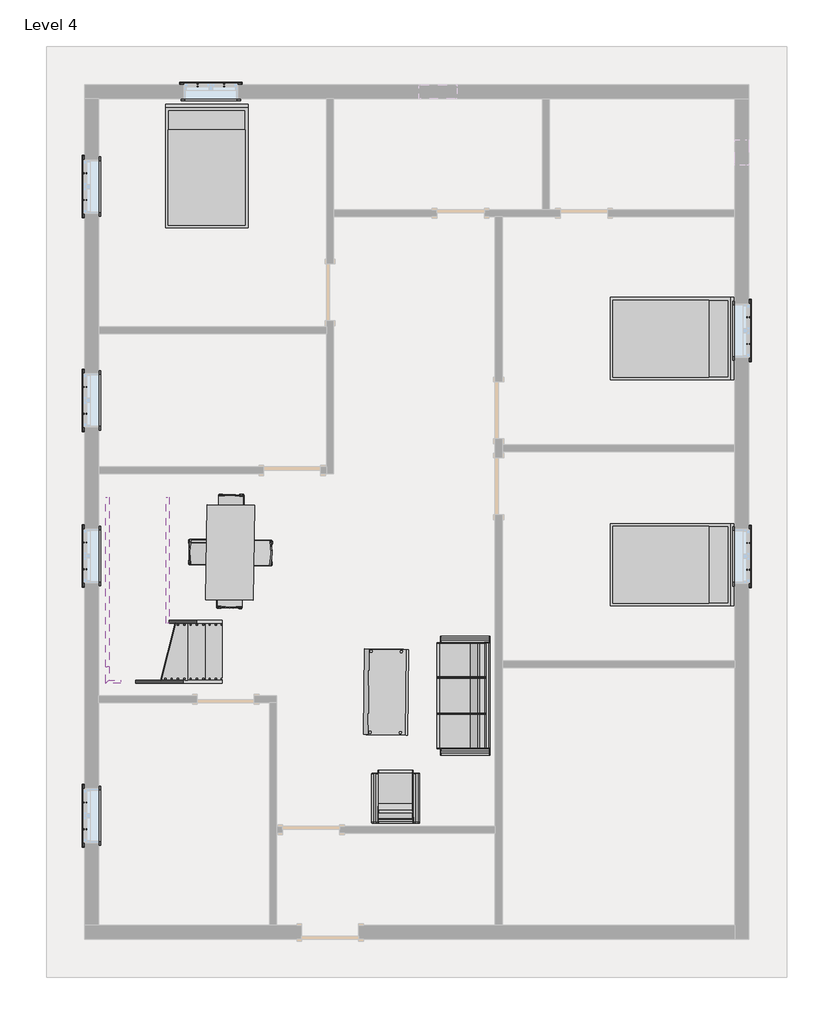
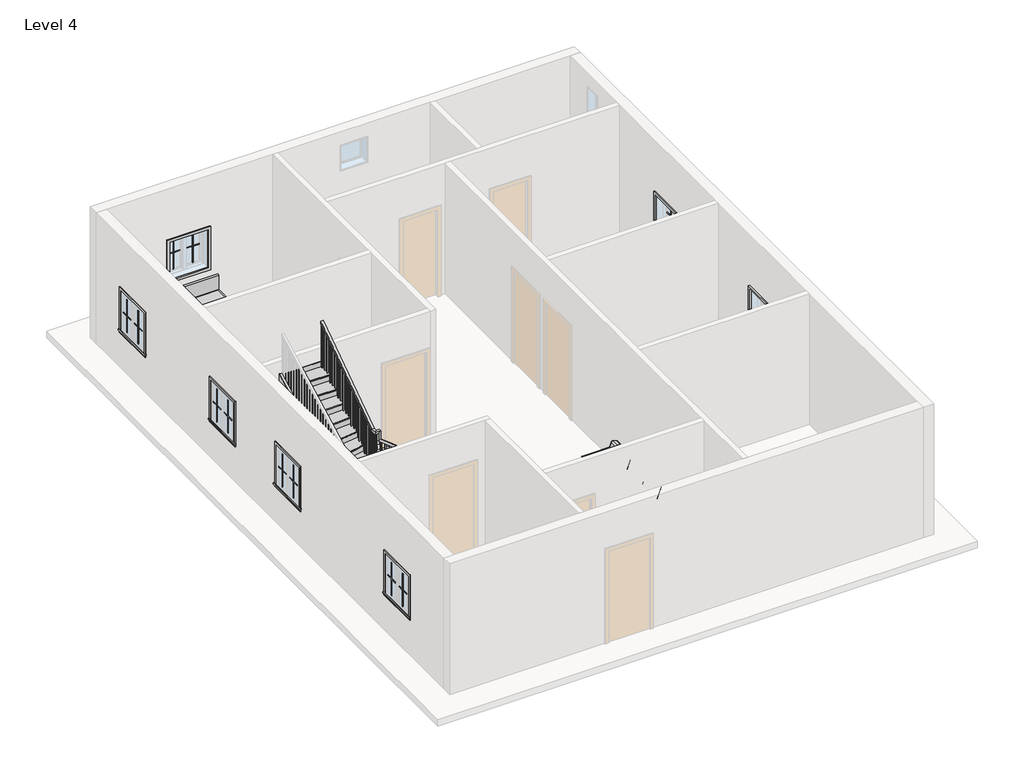
# One storey, part 2 of 2: 29 proxies, 6 furniture elements, 6 members, 1 railing, 1 stair flight.
"""IFC4 building model written with IfcOpenShell, lengths in millimetres."""

from ifc_helpers import new_model, si_unit, frame, origin, place, context, project, spatial, polyline, outline, extrude, faceted_brep, transform, mapped, element, save
from components import modern_coffee_table_17989_modern_coffee_table_17989_d3a860c8, muntin_pattern_2x2_muntin_pattern_2x2_b3fe6957, muntin_pattern_2x2_muntin_pattern_2x2_3e0ecaf2, trim_window_exterior_flat_with_sill_41619996, trim_window_interior_flat_picture_frame_51c85655, furniture_2fc85b74, furniture_29a9adb8, furniture_57072a26, furniture_f28dd14e, furniture_402a1f5e, bed_17739_bed_17739_15c61121, dining_table_w_chairs_11374_0cdfc61b, stair_flight_62476df0

model = new_model("IFC4")

# Units and contexts
model_context = context("Model", 3, world=origin())
ifc_project = project(units=[si_unit("LENGTHUNIT", "METRE", prefix="MILLI")], contexts=[model_context])

# Site, building, storey
site = spatial("IfcSite", under=ifc_project)
building = spatial("IfcBuilding", under=site)
storey = spatial("IfcBuildingStorey", under=building, Name="Level 4", Elevation=6400.8)

# Proxies
placement = place(None, origin())
modern_coffee_table_17989_modern_coffee_table_17989_shape = modern_coffee_table_17989_modern_coffee_table_17989_d3a860c8(model_context)
element("IfcBuildingElementProxy", 1, Name="Modern_Coffee_Table_17989 : Modern_Coffee_Table_17989", ObjectType="Modern_Coffee_Table_17989 : Modern_Coffee_Table_17989", at=placement, inside=storey, context=model_context, shape_type="MappedRepresentation", body=[
    mapped(modern_coffee_table_17989_modern_coffee_table_17989_shape, transform((-2106.8718825, -2116.758017, 6400.8), x_axis=(0.012591066442684793, 0.9999207293810025, 0.0), y_axis=(-0.9999207293810025, 0.012591066442684793, 0.0), z_axis=(0.0, 0.0, 1.0))),
])
muntin_pattern_2x2_muntin_pattern_2x2_shape = muntin_pattern_2x2_muntin_pattern_2x2_b3fe6957(model_context)
element("IfcBuildingElementProxy", 2, Name="Muntin Pattern_2x2 : Muntin Pattern_2x2", ObjectType="Muntin Pattern_2x2 : Muntin Pattern_2x2", at=placement, inside=storey, context=model_context, shape_type="MappedRepresentation", body=[
    mapped(muntin_pattern_2x2_muntin_pattern_2x2_shape, transform((-4775.9474931, 7386.6685985, 7385.05), x_axis=(1.0, 0.0, 0.0), y_axis=(0.0, 1.0, 0.0), z_axis=(0.0, 0.0, 1.0))),
])
element("IfcBuildingElementProxy", 3, Name="Muntin Pattern_2x2 : Muntin Pattern_2x2", ObjectType="Muntin Pattern_2x2 : Muntin Pattern_2x2", at=placement, inside=storey, context=model_context, shape_type="MappedRepresentation", body=[
    mapped(muntin_pattern_2x2_muntin_pattern_2x2_shape, transform((4068.0150069, 3660.8060985, 7385.05), x_axis=(0.0, -1.0, 0.0), y_axis=(1.0, 0.0, 0.0), z_axis=(0.0, 0.0, 1.0))),
])
element("IfcBuildingElementProxy", 4, Name="Muntin Pattern_2x2 : Muntin Pattern_2x2", ObjectType="Muntin Pattern_2x2 : Muntin Pattern_2x2", at=placement, inside=storey, context=model_context, shape_type="MappedRepresentation", body=[
    mapped(muntin_pattern_2x2_muntin_pattern_2x2_shape, transform((4068.0150069, 40.9802908, 7385.05), x_axis=(0.0, -1.0, 0.0), y_axis=(1.0, 0.0, 0.0), z_axis=(0.0, 0.0, 1.0))),
])
element("IfcBuildingElementProxy", 5, Name="Muntin Pattern_2x2 : Muntin Pattern_2x2", ObjectType="Muntin Pattern_2x2 : Muntin Pattern_2x2", at=placement, inside=storey, context=model_context, shape_type="MappedRepresentation", body=[
    mapped(muntin_pattern_2x2_muntin_pattern_2x2_shape, transform((-6580.9349931, 2114.5810985, 7385.05), x_axis=(0.0, 1.0, 0.0), y_axis=(-1.0, 0.0, 0.0), z_axis=(0.0, 0.0, 1.0))),
])
element("IfcBuildingElementProxy", 6, Name="Muntin Pattern_2x2 : Muntin Pattern_2x2", ObjectType="Muntin Pattern_2x2 : Muntin Pattern_2x2", at=placement, inside=storey, context=model_context, shape_type="MappedRepresentation", body=[
    mapped(muntin_pattern_2x2_muntin_pattern_2x2_shape, transform((-6580.9349931, 5543.5810985, 7385.05), x_axis=(0.0, 1.0, 0.0), y_axis=(-1.0, 0.0, 0.0), z_axis=(0.0, 0.0, 1.0))),
])
element("IfcBuildingElementProxy", 7, Name="Muntin Pattern_2x2 : Muntin Pattern_2x2", ObjectType="Muntin Pattern_2x2 : Muntin Pattern_2x2", at=placement, inside=storey, context=model_context, shape_type="MappedRepresentation", body=[
    mapped(muntin_pattern_2x2_muntin_pattern_2x2_shape, transform((-6580.9349931, -4549.7439015, 7385.05), x_axis=(0.0, 1.0, 0.0), y_axis=(-1.0, 0.0, 0.0), z_axis=(0.0, 0.0, 1.0))),
])
element("IfcBuildingElementProxy", 8, Name="Muntin Pattern_2x2 : Muntin Pattern_2x2", ObjectType="Muntin Pattern_2x2 : Muntin Pattern_2x2", at=placement, inside=storey, context=model_context, shape_type="MappedRepresentation", body=[
    mapped(muntin_pattern_2x2_muntin_pattern_2x2_shape, transform((-6580.9349931, -380.9689015, 7385.05), x_axis=(0.0, 1.0, 0.0), y_axis=(-1.0, 0.0, 0.0), z_axis=(0.0, 0.0, 1.0))),
])
muntin_pattern_2x2_muntin_pattern_2x2_2_shape = muntin_pattern_2x2_muntin_pattern_2x2_3e0ecaf2(model_context)
element("IfcBuildingElementProxy", 9, Name="Muntin Pattern_2x2 : Muntin Pattern_2x2", ObjectType="Muntin Pattern_2x2 : Muntin Pattern_2x2", at=placement, inside=storey, context=model_context, shape_type="MappedRepresentation", body=[
    mapped(muntin_pattern_2x2_muntin_pattern_2x2_2_shape, transform((-4347.3224931, 7386.6685985, 7385.05), x_axis=(-1.0, 0.0, 0.0), y_axis=(0.0, -1.0, 0.0), z_axis=(0.0, 0.0, 1.0))),
])
element("IfcBuildingElementProxy", 10, Name="Muntin Pattern_2x2 : Muntin Pattern_2x2", ObjectType="Muntin Pattern_2x2 : Muntin Pattern_2x2", at=placement, inside=storey, context=model_context, shape_type="MappedRepresentation", body=[
    mapped(muntin_pattern_2x2_muntin_pattern_2x2_2_shape, transform((4068.0150069, 3232.1810985, 7385.05), x_axis=(0.0, 1.0, 0.0), y_axis=(-1.0, 0.0, 0.0), z_axis=(0.0, 0.0, 1.0))),
])
element("IfcBuildingElementProxy", 11, Name="Muntin Pattern_2x2 : Muntin Pattern_2x2", ObjectType="Muntin Pattern_2x2 : Muntin Pattern_2x2", at=placement, inside=storey, context=model_context, shape_type="MappedRepresentation", body=[
    mapped(muntin_pattern_2x2_muntin_pattern_2x2_2_shape, transform((4068.0150069, -387.6447092, 7385.05), x_axis=(0.0, 1.0, 0.0), y_axis=(-1.0, 0.0, 0.0), z_axis=(0.0, 0.0, 1.0))),
])
element("IfcBuildingElementProxy", 12, Name="Muntin Pattern_2x2 : Muntin Pattern_2x2", ObjectType="Muntin Pattern_2x2 : Muntin Pattern_2x2", at=placement, inside=storey, context=model_context, shape_type="MappedRepresentation", body=[
    mapped(muntin_pattern_2x2_muntin_pattern_2x2_2_shape, transform((-6580.9349931, 2543.2060985, 7385.05), x_axis=(0.0, -1.0, 0.0), y_axis=(1.0, 0.0, 0.0), z_axis=(0.0, 0.0, 1.0))),
])
element("IfcBuildingElementProxy", 13, Name="Muntin Pattern_2x2 : Muntin Pattern_2x2", ObjectType="Muntin Pattern_2x2 : Muntin Pattern_2x2", at=placement, inside=storey, context=model_context, shape_type="MappedRepresentation", body=[
    mapped(muntin_pattern_2x2_muntin_pattern_2x2_2_shape, transform((-6580.9349931, 5972.2060985, 7385.05), x_axis=(0.0, -1.0, 0.0), y_axis=(1.0, 0.0, 0.0), z_axis=(0.0, 0.0, 1.0))),
])
element("IfcBuildingElementProxy", 14, Name="Muntin Pattern_2x2 : Muntin Pattern_2x2", ObjectType="Muntin Pattern_2x2 : Muntin Pattern_2x2", at=placement, inside=storey, context=model_context, shape_type="MappedRepresentation", body=[
    mapped(muntin_pattern_2x2_muntin_pattern_2x2_2_shape, transform((-6580.9349931, -4121.1189015, 7385.05), x_axis=(0.0, -1.0, 0.0), y_axis=(1.0, 0.0, 0.0), z_axis=(0.0, 0.0, 1.0))),
])
element("IfcBuildingElementProxy", 15, Name="Muntin Pattern_2x2 : Muntin Pattern_2x2", ObjectType="Muntin Pattern_2x2 : Muntin Pattern_2x2", at=placement, inside=storey, context=model_context, shape_type="MappedRepresentation", body=[
    mapped(muntin_pattern_2x2_muntin_pattern_2x2_2_shape, transform((-6580.9349931, 47.6560985, 7385.05), x_axis=(0.0, -1.0, 0.0), y_axis=(1.0, 0.0, 0.0), z_axis=(0.0, 0.0, 1.0))),
])
trim_window_exterior_flat_with_sill_shape = trim_window_exterior_flat_with_sill_41619996(model_context)
element("IfcBuildingElementProxy", 16, Name="Trim-Window-Exterior-Flat : with Sill", ObjectType="Trim-Window-Exterior-Flat : with Sill", at=placement, inside=storey, context=model_context, shape_type="MappedRepresentation", body=[
    mapped(trim_window_exterior_flat_with_sill_shape, transform((-4561.6349931, 7396.1935985, 8229.6), x_axis=(-1.0, 0.0, 0.0), y_axis=(0.0, 0.0, 1.0), z_axis=(0.0, 1.0, 0.0))),
])
element("IfcBuildingElementProxy", 17, Name="Trim-Window-Exterior-Flat : with Sill", ObjectType="Trim-Window-Exterior-Flat : with Sill", at=placement, inside=storey, context=model_context, shape_type="MappedRepresentation", body=[
    mapped(trim_window_exterior_flat_with_sill_shape, transform((4077.5400069, 3446.4935985, 8229.6), x_axis=(0.0, 1.0, 0.0), y_axis=(0.0, 0.0, 1.0), z_axis=(1.0, 0.0, 0.0))),
])
element("IfcBuildingElementProxy", 18, Name="Trim-Window-Exterior-Flat : with Sill", ObjectType="Trim-Window-Exterior-Flat : with Sill", at=placement, inside=storey, context=model_context, shape_type="MappedRepresentation", body=[
    mapped(trim_window_exterior_flat_with_sill_shape, transform((4077.5400069, -173.3322092, 8229.6), x_axis=(0.0, 1.0, 0.0), y_axis=(0.0, 0.0, 1.0), z_axis=(1.0, 0.0, 0.0))),
])
element("IfcBuildingElementProxy", 19, Name="Trim-Window-Exterior-Flat : with Sill", ObjectType="Trim-Window-Exterior-Flat : with Sill", at=placement, inside=storey, context=model_context, shape_type="MappedRepresentation", body=[
    mapped(trim_window_exterior_flat_with_sill_shape, transform((-6590.4599931, 2328.8935985, 8229.6), x_axis=(0.0, -1.0, 0.0), y_axis=(0.0, 0.0, 1.0), z_axis=(-1.0, 0.0, 0.0))),
])
element("IfcBuildingElementProxy", 20, Name="Trim-Window-Exterior-Flat : with Sill", ObjectType="Trim-Window-Exterior-Flat : with Sill", at=placement, inside=storey, context=model_context, shape_type="MappedRepresentation", body=[
    mapped(trim_window_exterior_flat_with_sill_shape, transform((-6590.4599931, 5757.8935985, 8229.6), x_axis=(0.0, -1.0, 0.0), y_axis=(0.0, 0.0, 1.0), z_axis=(-1.0, 0.0, 0.0))),
])
element("IfcBuildingElementProxy", 21, Name="Trim-Window-Exterior-Flat : with Sill", ObjectType="Trim-Window-Exterior-Flat : with Sill", at=placement, inside=storey, context=model_context, shape_type="MappedRepresentation", body=[
    mapped(trim_window_exterior_flat_with_sill_shape, transform((-6590.4599931, -4335.4314015, 8229.6), x_axis=(0.0, -1.0, 0.0), y_axis=(0.0, 0.0, 1.0), z_axis=(-1.0, 0.0, 0.0))),
])
element("IfcBuildingElementProxy", 22, Name="Trim-Window-Exterior-Flat : with Sill", ObjectType="Trim-Window-Exterior-Flat : with Sill", at=placement, inside=storey, context=model_context, shape_type="MappedRepresentation", body=[
    mapped(trim_window_exterior_flat_with_sill_shape, transform((-6590.4599931, -166.6564015, 8229.6), x_axis=(0.0, -1.0, 0.0), y_axis=(0.0, 0.0, 1.0), z_axis=(-1.0, 0.0, 0.0))),
])
trim_window_interior_flat_picture_frame_shape = trim_window_interior_flat_picture_frame_51c85655(model_context)
element("IfcBuildingElementProxy", 23, Name="Trim-Window-Interior-Flat : Picture Frame", ObjectType="Trim-Window-Interior-Flat : Picture Frame", at=placement, inside=storey, context=model_context, shape_type="MappedRepresentation", body=[
    mapped(trim_window_interior_flat_picture_frame_shape, transform((-4561.6349931, 7167.5935985, 8229.6), x_axis=(1.0, 0.0, 0.0), y_axis=(0.0, 0.0, 1.0), z_axis=(0.0, -1.0, 0.0))),
])
element("IfcBuildingElementProxy", 24, Name="Trim-Window-Interior-Flat : Picture Frame", ObjectType="Trim-Window-Interior-Flat : Picture Frame", at=placement, inside=storey, context=model_context, shape_type="MappedRepresentation", body=[
    mapped(trim_window_interior_flat_picture_frame_shape, transform((3848.9400069, 3446.4935985, 8229.6), x_axis=(0.0, -1.0, 0.0), y_axis=(0.0, 0.0, 1.0), z_axis=(-1.0, 0.0, 0.0))),
])
element("IfcBuildingElementProxy", 25, Name="Trim-Window-Interior-Flat : Picture Frame", ObjectType="Trim-Window-Interior-Flat : Picture Frame", at=placement, inside=storey, context=model_context, shape_type="MappedRepresentation", body=[
    mapped(trim_window_interior_flat_picture_frame_shape, transform((3848.9400069, -173.3322092, 8229.6), x_axis=(0.0, -1.0, 0.0), y_axis=(0.0, 0.0, 1.0), z_axis=(-1.0, 0.0, 0.0))),
])
element("IfcBuildingElementProxy", 26, Name="Trim-Window-Interior-Flat : Picture Frame", ObjectType="Trim-Window-Interior-Flat : Picture Frame", at=placement, inside=storey, context=model_context, shape_type="MappedRepresentation", body=[
    mapped(trim_window_interior_flat_picture_frame_shape, transform((-6361.8599931, 2328.8935985, 8229.6), x_axis=(0.0, 1.0, 0.0), y_axis=(0.0, 0.0, 1.0), z_axis=(1.0, 0.0, 0.0))),
])
element("IfcBuildingElementProxy", 27, Name="Trim-Window-Interior-Flat : Picture Frame", ObjectType="Trim-Window-Interior-Flat : Picture Frame", at=placement, inside=storey, context=model_context, shape_type="MappedRepresentation", body=[
    mapped(trim_window_interior_flat_picture_frame_shape, transform((-6361.8599931, 5757.8935985, 8229.6), x_axis=(0.0, 1.0, 0.0), y_axis=(0.0, 0.0, 1.0), z_axis=(1.0, 0.0, 0.0))),
])
element("IfcBuildingElementProxy", 28, Name="Trim-Window-Interior-Flat : Picture Frame", ObjectType="Trim-Window-Interior-Flat : Picture Frame", at=placement, inside=storey, context=model_context, shape_type="MappedRepresentation", body=[
    mapped(trim_window_interior_flat_picture_frame_shape, transform((-6361.8599931, -4335.4314015, 8229.6), x_axis=(0.0, 1.0, 0.0), y_axis=(0.0, 0.0, 1.0), z_axis=(1.0, 0.0, 0.0))),
])
element("IfcBuildingElementProxy", 29, Name="Trim-Window-Interior-Flat : Picture Frame", ObjectType="Trim-Window-Interior-Flat : Picture Frame", at=placement, inside=storey, context=model_context, shape_type="MappedRepresentation", body=[
    mapped(trim_window_interior_flat_picture_frame_shape, transform((-6361.8599931, -166.6564015, 8229.6), x_axis=(0.0, 1.0, 0.0), y_axis=(0.0, 0.0, 1.0), z_axis=(1.0, 0.0, 0.0))),
])

# Furniture
furniture_shape = furniture_2fc85b74(model_context)
furniture_2_shape = furniture_29a9adb8(model_context)
furniture_3_shape = furniture_57072a26(model_context)
element("IfcFurniture", 30, at=placement, inside=storey, context=model_context, shape_type="MappedRepresentation", body=[
    mapped(furniture_shape, transform((-877.7263413, -2408.2064015, 6400.8), x_axis=(0.0, -1.0, 0.0), y_axis=(1.0, 0.0, 0.0), z_axis=(0.0, 0.0, 1.0))),
    mapped(furniture_2_shape, transform((-877.7263413, -2408.2064015, 6400.8), x_axis=(0.0, -1.0, 0.0), y_axis=(1.0, 0.0, 0.0), z_axis=(0.0, 0.0, 1.0))),
    mapped(furniture_3_shape, transform((-877.7263413, -2408.2064015, 6400.8), x_axis=(0.0, -1.0, 0.0), y_axis=(1.0, 0.0, 0.0), z_axis=(0.0, 0.0, 1.0))),
])
furniture_4_shape = furniture_f28dd14e(model_context)
furniture_5_shape = furniture_402a1f5e(model_context)
element("IfcFurniture", 31, at=placement, inside=storey, context=model_context, shape_type="MappedRepresentation", body=[
    mapped(furniture_4_shape, transform((-1595.4975416, -3653.2527501, 6400.8), x_axis=(-1.0, 0.0, 0.0), y_axis=(0.0, -1.0, 0.0), z_axis=(0.0, 0.0, 1.0))),
    mapped(furniture_5_shape, transform((-1595.4975416, -3653.2527501, 6400.8), x_axis=(-1.0, 0.0, 0.0), y_axis=(0.0, -1.0, 0.0), z_axis=(0.0, 0.0, 1.0))),
])
bed_17739_bed_17739_shape = bed_17739_bed_17739_15c61121(model_context)
element("IfcFurniture", 32, ObjectType="Bed_17739 : Bed_17739", at=placement, inside=storey, context=model_context, shape_type="MappedRepresentation", body=[
    mapped(bed_17739_bed_17739_shape, transform((-4628.3099931, 6062.6935985, 6400.8), x_axis=(1.0, 0.0, 0.0), y_axis=(0.0, 1.0, 0.0), z_axis=(0.0, 0.0, 1.0))),
])
element("IfcFurniture", 33, ObjectType="Bed_17739 : Bed_17739", at=placement, inside=storey, context=model_context, shape_type="MappedRepresentation", body=[
    mapped(bed_17739_bed_17739_shape, transform((2820.2400069, 3319.4935985, 6400.8), x_axis=(0.0, -1.0, 0.0), y_axis=(1.0, 0.0, 0.0), z_axis=(0.0, 0.0, 1.0))),
])
element("IfcFurniture", 34, ObjectType="Bed_17739 : Bed_17739", at=placement, inside=storey, context=model_context, shape_type="MappedRepresentation", body=[
    mapped(bed_17739_bed_17739_shape, transform((2820.2400069, -307.008017, 6400.8), x_axis=(0.0, -1.0, 0.0), y_axis=(1.0, 0.0, 0.0), z_axis=(0.0, 0.0, 1.0))),
])
dining_table_w_chairs_11374_shape = dining_table_w_chairs_11374_0cdfc61b(model_context)
element("IfcFurniture", 35, ObjectType="Dining_Table_w_Chairs_11374", at=placement, inside=storey, context=model_context, shape_type="MappedRepresentation", body=[
    mapped(dining_table_w_chairs_11374_shape, transform((-4154.6586335, -131.9172641, 6400.8), x_axis=(0.015873758475140665, 0.9998740039584353, 0.0), y_axis=(-0.9998740039584353, 0.015873758475140665, 0.0), z_axis=(0.0, 0.0, 1.0))),
])

# Members
element("IfcMember", 36, ObjectType="Stringer - 2\" Width", at=placement, inside=storey, context=model_context, shape_type="SweptSolid", body=[
    extrude(outline(polyline([(6990.8562463, -4378.4230036), (7323.6849999, -4378.4230036), (8038.8971411, -6009.0851964), (7706.0683876, -6009.0851964), (6990.8562463, -4378.4230036)])), frame((0.0, -2211.3564015, 0.0), z_axis=(0.0, 1.0, 0.0), x_axis=(0.0, 0.0, 1.0)), (0.0, 0.0, 1.0), 50.8),
])
element("IfcMember", 37, ObjectType="Stringer - 2\" Width", at=placement, inside=storey, context=model_context, shape_type="SweptSolid", body=[
    extrude(outline(polyline([(-6009.0851964, -2160.5564015), (-6009.0851964, -2211.3564015), (-6247.5599931, -2211.3564015), (-6196.7599931, -2160.5564015), (-6009.0851964, -2160.5564015)])), frame((0.0, 0.0, 7706.0683876), z_axis=(0.0, 0.0, 1.0), x_axis=(1.0, 0.0, 0.0)), (0.0, 0.0, 1.0), 332.8287535),
])
element("IfcMember", 38, ObjectType="Stringer - 2\" Width", at=placement, inside=storey, context=model_context, shape_type="SweptSolid", body=[
    extrude(outline(polyline([(-6196.7599931, -2160.5564015), (-6247.5599931, -2211.3564015), (-6247.5599931, -1942.4030584), (-6196.7599931, -1942.4030584), (-6196.7599931, -2160.5564015)])), frame((0.0, 0.0, 7706.0683876), z_axis=(0.0, 0.0, 1.0), x_axis=(1.0, 0.0, 0.0)), (0.0, 0.0, 1.0), 332.8287535),
])
element("IfcMember", 39, ObjectType="Stringer - 2\" Width", at=placement, inside=storey, context=model_context, shape_type="SweptSolid", body=[
    extrude(outline(polyline([(-1942.4030584, 7706.0683876), (-1942.4030584, 8038.8971411), (775.380588, 9454.4189504), (775.380588, 9121.5901969), (-1942.4030584, 7706.0683876)])), frame((-6247.5599931, 0.0, 0.0), z_axis=(1.0, 0.0, 0.0), x_axis=(0.0, 1.0, 0.0)), (0.0, 0.0, 1.0), 50.8),
])
element("IfcMember", 40, ObjectType="Stringer - 2\" Width", at=placement, inside=storey, context=model_context, shape_type="SweptSolid", body=[
    extrude(outline(polyline([(6836.2922729, -4378.4230036), (7243.434734, -4378.4230036), (7998.9690344, -5231.5599931), (7591.8265733, -5231.5599931), (6836.2922729, -4378.4230036)])), frame((0.0, -1246.1564015, 0.0), z_axis=(0.0, 1.0, 0.0), x_axis=(0.0, 0.0, 1.0)), (0.0, 0.0, 1.0), 50.8),
])
element("IfcMember", 41, ObjectType="Stringer - 2\" Width", at=placement, inside=storey, context=model_context, shape_type="SweptSolid", body=[
    extrude(outline(polyline([(-1246.1564015, 7738.5212805), (-1246.1564015, 8110.7296678), (775.380588, 9527.5693854), (775.380588, 9155.3609981), (-1246.1564015, 7738.5212805)])), frame((-5282.3599931, 0.0, 0.0), z_axis=(1.0, 0.0, 0.0), x_axis=(0.0, 1.0, 0.0)), (0.0, 0.0, 1.0), 50.8),
])

# Railing
element("IfcRailing", 42, ObjectType="Handrail - Rectangular", at=placement, inside=storey, context=model_context, shape_type="SolidModel", body=[
    faceted_brep([(-4378.4230036, -1296.9564015, 8161.8666667), (-4378.4230036, -1296.9564015, 8096.9997378), (-4378.4230036, -1246.1564015, 8096.9997378), (-4378.4230036, -1246.1564015, 8161.8666667), (-5206.1599931, -1296.9564015, 8819.1201542), (-5256.9599931, -1296.9564015, 8794.590286), (-5256.9599931, -1246.1564015, 8794.590286), (-5206.1599931, -1246.1564015, 8819.1201542), (-5206.1599931, -1296.9564015, 9025.9172738), (-5256.9599931, -1296.9564015, 8975.1172738), (-5256.9599931, -1246.1564015, 8975.1172738), (-5206.1599931, -1246.1564015, 9025.9172738), (-5333.1599931, -1296.9564015, 9025.9172738), (-5333.1599931, -1296.9564015, 8975.1172738), (-5282.3599931, -1246.1564015, 8975.1172738), (-5282.3599931, -1246.1564015, 9025.9172738), (-5333.1599931, -1169.9564015, 9025.9172738), (-5333.1599931, -1154.1797661, 8975.1172738), (-5282.3599931, -1154.1797661, 8975.1172738), (-5282.3599931, -1169.9564015, 9025.9172738), (-5333.1599931, 775.380588, 10363.2), (-5282.3599931, 775.380588, 10363.2), (-5282.3599931, 775.380588, 10301.5546698), (-5333.1599931, 775.380588, 10301.5546698)], [[[0, 1, 2, 3]], [[1, 0, 4, 5]], [[2, 1, 5, 6]], [[3, 2, 6, 7]], [[0, 3, 7, 4]], [[5, 4, 8, 9]], [[6, 5, 9, 10]], [[7, 6, 10, 11]], [[4, 7, 11, 8]], [[9, 8, 12, 13]], [[10, 9, 13, 14]], [[11, 10, 14, 15]], [[8, 11, 15, 12]], [[13, 12, 16, 17]], [[14, 13, 17, 18]], [[15, 14, 18, 19]], [[12, 15, 19, 16]], [[20, 21, 22, 23]], [[17, 16, 20, 23]], [[18, 17, 23, 22]], [[19, 18, 22, 21]], [[16, 19, 21, 20]]]),
    extrude(outline(polyline([(750.9185985, 10284.7387679), (769.9685985, 10297.8343066), (769.9685985, 9279.4666667), (750.9185985, 9279.4666667), (750.9185985, 10284.7387679)])), frame((-5317.2849931, 0.0, 0.0), z_axis=(1.0, 0.0, 0.0), x_axis=(0.0, 1.0, 0.0)), (0.0, 0.0, 1.0), 19.05),
    extrude(outline(polyline([(649.3185985, 10214.8958945), (668.3685985, 10227.9914333), (668.3685985, 9279.4666667), (649.3185985, 9279.4666667), (649.3185985, 10214.8958945)])), frame((-5317.2849931, 0.0, 0.0), z_axis=(1.0, 0.0, 0.0), x_axis=(0.0, 1.0, 0.0)), (0.0, 0.0, 1.0), 19.05),
    extrude(outline(polyline([(547.7185985, 10145.0530212), (566.7685985, 10158.1485599), (566.7685985, 9279.4666667), (547.7185985, 9279.4666667), (547.7185985, 10145.0530212)])), frame((-5317.2849931, 0.0, 0.0), z_axis=(1.0, 0.0, 0.0), x_axis=(0.0, 1.0, 0.0)), (0.0, 0.0, 1.0), 19.05),
    extrude(outline(polyline([(446.1185985, 10075.2101478), (465.1685985, 10088.3056866), (465.1685985, 9110.1333333), (446.1185985, 9110.1333333), (446.1185985, 10075.2101478)])), frame((-5317.2849931, 0.0, 0.0), z_axis=(1.0, 0.0, 0.0), x_axis=(0.0, 1.0, 0.0)), (0.0, 0.0, 1.0), 19.05),
    extrude(outline(polyline([(344.5185985, 10005.3672745), (363.5685985, 10018.4628132), (363.5685985, 9110.1333333), (344.5185985, 9110.1333333), (344.5185985, 10005.3672745)])), frame((-5317.2849931, 0.0, 0.0), z_axis=(1.0, 0.0, 0.0), x_axis=(0.0, 1.0, 0.0)), (0.0, 0.0, 1.0), 19.05),
    extrude(outline(polyline([(242.9185985, 9935.5244011), (261.9685985, 9948.6199399), (261.9685985, 9110.1333333), (242.9185985, 9110.1333333), (242.9185985, 9935.5244011)])), frame((-5317.2849931, 0.0, 0.0), z_axis=(1.0, 0.0, 0.0), x_axis=(0.0, 1.0, 0.0)), (0.0, 0.0, 1.0), 19.05),
    extrude(outline(polyline([(141.3185985, 9865.6815278), (160.3685985, 9878.7770665), (160.3685985, 8940.8), (141.3185985, 8940.8), (141.3185985, 9865.6815278)])), frame((-5317.2849931, 0.0, 0.0), z_axis=(1.0, 0.0, 0.0), x_axis=(0.0, 1.0, 0.0)), (0.0, 0.0, 1.0), 19.05),
    extrude(outline(polyline([(39.7185985, 9795.8386544), (58.7685985, 9808.9341932), (58.7685985, 8940.8), (39.7185985, 8940.8), (39.7185985, 9795.8386544)])), frame((-5317.2849931, 0.0, 0.0), z_axis=(1.0, 0.0, 0.0), x_axis=(0.0, 1.0, 0.0)), (0.0, 0.0, 1.0), 19.05),
    extrude(outline(polyline([(-61.8814015, 9725.9957811), (-42.8314015, 9739.0913198), (-42.8314015, 8771.4666667), (-61.8814015, 8771.4666667), (-61.8814015, 9725.9957811)])), frame((-5317.2849931, 0.0, 0.0), z_axis=(1.0, 0.0, 0.0), x_axis=(0.0, 1.0, 0.0)), (0.0, 0.0, 1.0), 19.05),
    extrude(outline(polyline([(-163.4814015, 9656.1529077), (-144.4314015, 9669.2484465), (-144.4314015, 8771.4666667), (-163.4814015, 8771.4666667), (-163.4814015, 9656.1529077)])), frame((-5317.2849931, 0.0, 0.0), z_axis=(1.0, 0.0, 0.0), x_axis=(0.0, 1.0, 0.0)), (0.0, 0.0, 1.0), 19.05),
    extrude(outline(polyline([(-265.0814015, 9586.3100344), (-246.0314015, 9599.4055731), (-246.0314015, 8771.4666667), (-265.0814015, 8771.4666667), (-265.0814015, 9586.3100344)])), frame((-5317.2849931, 0.0, 0.0), z_axis=(1.0, 0.0, 0.0), x_axis=(0.0, 1.0, 0.0)), (0.0, 0.0, 1.0), 19.05),
    extrude(outline(polyline([(-366.6814015, 9516.467161), (-347.6314015, 9529.5626998), (-347.6314015, 8602.1333333), (-366.6814015, 8602.1333333), (-366.6814015, 9516.467161)])), frame((-5317.2849931, 0.0, 0.0), z_axis=(1.0, 0.0, 0.0), x_axis=(0.0, 1.0, 0.0)), (0.0, 0.0, 1.0), 19.05),
    extrude(outline(polyline([(-468.2814015, 9446.6242877), (-449.2314015, 9459.7198264), (-449.2314015, 8602.1333333), (-468.2814015, 8602.1333333), (-468.2814015, 9446.6242877)])), frame((-5317.2849931, 0.0, 0.0), z_axis=(1.0, 0.0, 0.0), x_axis=(0.0, 1.0, 0.0)), (0.0, 0.0, 1.0), 19.05),
    extrude(outline(polyline([(-569.8814015, 9376.7814143), (-550.8314015, 9389.8769531), (-550.8314015, 8602.1333333), (-569.8814015, 8602.1333333), (-569.8814015, 9376.7814143)])), frame((-5317.2849931, 0.0, 0.0), z_axis=(1.0, 0.0, 0.0), x_axis=(0.0, 1.0, 0.0)), (0.0, 0.0, 1.0), 19.05),
    extrude(outline(polyline([(-671.4814015, 9306.938541), (-652.4314015, 9320.0340797), (-652.4314015, 8432.8), (-671.4814015, 8432.8), (-671.4814015, 9306.938541)])), frame((-5317.2849931, 0.0, 0.0), z_axis=(1.0, 0.0, 0.0), x_axis=(0.0, 1.0, 0.0)), (0.0, 0.0, 1.0), 19.05),
    extrude(outline(polyline([(-773.0814015, 9237.0956676), (-754.0314015, 9250.1912064), (-754.0314015, 8432.8), (-773.0814015, 8432.8), (-773.0814015, 9237.0956676)])), frame((-5317.2849931, 0.0, 0.0), z_axis=(1.0, 0.0, 0.0), x_axis=(0.0, 1.0, 0.0)), (0.0, 0.0, 1.0), 19.05),
    extrude(outline(polyline([(-874.6814015, 9167.2527943), (-855.6314015, 9180.348333), (-855.6314015, 8263.4666667), (-874.6814015, 8263.4666667), (-874.6814015, 9167.2527943)])), frame((-5317.2849931, 0.0, 0.0), z_axis=(1.0, 0.0, 0.0), x_axis=(0.0, 1.0, 0.0)), (0.0, 0.0, 1.0), 19.05),
    extrude(outline(polyline([(-976.2814015, 9097.4099209), (-957.2314015, 9110.5054597), (-957.2314015, 8263.4666667), (-976.2814015, 8263.4666667), (-976.2814015, 9097.4099209)])), frame((-5317.2849931, 0.0, 0.0), z_axis=(1.0, 0.0, 0.0), x_axis=(0.0, 1.0, 0.0)), (0.0, 0.0, 1.0), 19.05),
    extrude(outline(polyline([(-1077.8814015, 9027.5670476), (-1058.8314015, 9040.6625863), (-1058.8314015, 8094.1333333), (-1077.8814015, 8094.1333333), (-1077.8814015, 9027.5670476)])), frame((-5317.2849931, 0.0, 0.0), z_axis=(1.0, 0.0, 0.0), x_axis=(0.0, 1.0, 0.0)), (0.0, 0.0, 1.0), 19.05),
    extrude(outline(polyline([(-1179.4814015, 8957.7241742), (-1160.4314015, 8970.819713), (-1160.4314015, 8094.1333333), (-1179.4814015, 8094.1333333), (-1179.4814015, 8957.7241742)])), frame((-5317.2849931, 0.0, 0.0), z_axis=(1.0, 0.0, 0.0), x_axis=(0.0, 1.0, 0.0)), (0.0, 0.0, 1.0), 19.05),
    extrude(outline(polyline([(-5283.2980036, -1262.0314015), (-5283.2980036, -1281.0814015), (-5302.3480036, -1281.0814015), (-5302.3480036, -1262.0314015), (-5283.2980036, -1262.0314015)])), frame((0.0, 0.0, 7924.8), z_axis=(0.0, 0.0, 1.0), x_axis=(1.0, 0.0, 0.0)), (0.0, 0.0, 1.0), 1050.3172738),
    extrude(outline(polyline([(8734.8295097, -5181.6980036), (8749.9559074, -5200.7480036), (7755.4666667, -5200.7480036), (7755.4666667, -5181.6980036), (8734.8295097, -5181.6980036)])), frame((0.0, -1281.0814015, 0.0), z_axis=(0.0, 1.0, 0.0), x_axis=(0.0, 0.0, 1.0)), (0.0, 0.0, 1.0), 19.05),
    extrude(outline(polyline([(8654.1553883, -5080.0980036), (8669.2817861, -5099.1480036), (7586.1333333, -5099.1480036), (7586.1333333, -5080.0980036), (8654.1553883, -5080.0980036)])), frame((0.0, -1281.0814015, 0.0), z_axis=(0.0, 1.0, 0.0), x_axis=(0.0, 0.0, 1.0)), (0.0, 0.0, 1.0), 19.05),
    extrude(outline(polyline([(8573.481267, -4978.4980036), (8588.6076647, -4997.5480036), (7586.1333333, -4997.5480036), (7586.1333333, -4978.4980036), (8573.481267, -4978.4980036)])), frame((0.0, -1281.0814015, 0.0), z_axis=(0.0, 1.0, 0.0), x_axis=(0.0, 0.0, 1.0)), (0.0, 0.0, 1.0), 19.05),
    extrude(outline(polyline([(8492.8071456, -4876.8980036), (8507.9335434, -4895.9480036), (7416.8, -4895.9480036), (7416.8, -4876.8980036), (8492.8071456, -4876.8980036)])), frame((0.0, -1281.0814015, 0.0), z_axis=(0.0, 1.0, 0.0), x_axis=(0.0, 0.0, 1.0)), (0.0, 0.0, 1.0), 19.05),
    extrude(outline(polyline([(8412.1330243, -4775.2980036), (8427.259422, -4794.3480036), (7416.8, -4794.3480036), (7416.8, -4775.2980036), (8412.1330243, -4775.2980036)])), frame((0.0, -1281.0814015, 0.0), z_axis=(0.0, 1.0, 0.0), x_axis=(0.0, 0.0, 1.0)), (0.0, 0.0, 1.0), 19.05),
    extrude(outline(polyline([(8331.4589029, -4673.6980036), (8346.5853007, -4692.7480036), (7416.8, -4692.7480036), (7416.8, -4673.6980036), (8331.4589029, -4673.6980036)])), frame((0.0, -1281.0814015, 0.0), z_axis=(0.0, 1.0, 0.0), x_axis=(0.0, 0.0, 1.0)), (0.0, 0.0, 1.0), 19.05),
    extrude(outline(polyline([(8250.7847816, -4572.0980036), (8265.9111793, -4591.1480036), (7247.4666667, -4591.1480036), (7247.4666667, -4572.0980036), (8250.7847816, -4572.0980036)])), frame((0.0, -1281.0814015, 0.0), z_axis=(0.0, 1.0, 0.0), x_axis=(0.0, 0.0, 1.0)), (0.0, 0.0, 1.0), 19.05),
    extrude(outline(polyline([(8170.1106602, -4470.4980036), (8185.237058, -4489.5480036), (7247.4666667, -4489.5480036), (7247.4666667, -4470.4980036), (8170.1106602, -4470.4980036)])), frame((0.0, -1281.0814015, 0.0), z_axis=(0.0, 1.0, 0.0), x_axis=(0.0, 0.0, 1.0)), (0.0, 0.0, 1.0), 19.05),
    extrude(outline(polyline([(-5298.2349931, -1262.0314015), (-5298.2349931, -1281.0814015), (-5317.2849931, -1281.0814015), (-5317.2849931, -1262.0314015), (-5298.2349931, -1262.0314015)])), frame((0.0, 0.0, 7924.8), z_axis=(0.0, 0.0, 1.0), x_axis=(1.0, 0.0, 0.0)), (0.0, 0.0, 1.0), 1050.3172738),
    extrude(outline(polyline([(756.330588, 10288.459131), (775.380588, 10301.5546698), (775.380588, 9279.4666667), (756.330588, 9279.4666667), (756.330588, 10288.459131)])), frame((-5317.2849931, 0.0, 0.0), z_axis=(1.0, 0.0, 0.0), x_axis=(0.0, 1.0, 0.0)), (0.0, 0.0, 1.0), 19.05),
    extrude(outline(polyline([(8096.9997378, -4378.4230036), (8112.1261355, -4397.4730036), (7247.4666667, -4397.4730036), (7247.4666667, -4378.4230036), (8096.9997378, -4378.4230036)])), frame((0.0, -1281.0814015, 0.0), z_axis=(0.0, 1.0, 0.0), x_axis=(0.0, 0.0, 1.0)), (0.0, 0.0, 1.0), 19.05),
])

# Stair flight
stair_flight_shape = stair_flight_62476df0(model_context)
element("IfcStairFlight", 43, ObjectType="2\" Tread 1\" Nosing 1/4\" Riser", at=placement, inside=storey, context=model_context, shape_type="MappedRepresentation", body=[
    mapped(stair_flight_shape, transform((0.0, 0.0, 0.0), x_axis=(1.0, 0.0, 0.0), y_axis=(0.0, 1.0, 0.0), z_axis=(0.0, 0.0, 1.0))),
])

save(model, "model.ifc")

# Revit data of these elements
# Type "Modern_Coffee_Table_17989 : Modern_Coffee_Table_17989"
#   Default Elevation = 0
# Type "Muntin Pattern_2x2 : Muntin Pattern_2x2"
#   Width [instance default] = 4' - 0"
#   Thickness = 0' - 0 1/2"
#   Height [instance default] = 4' - 0"
#   Distance = 0' - 0 3/4"
#   Interior Material [instance default] = none
#   Exterior Material [instance default] = none
#   Default Elevation = 0
# Type "Trim-Window-Exterior-Flat : with Sill"
#   Trim Width = 0' - 2 1/4"
#   Trim Thickness_Picture Frame = 0' - 1 1/4"
#   Trim Thickness_with Sill = 0' - 0 3/4"
#   Sill Thickness = 0' - 1 1/4"
#   Opening Width [instance default] = 2' - 0"
#   Opening Height [instance default] = 3' - 0"
#   Default Elevation = 4' - 0"
#   Sill = yes
#   Picture Frame = no
#   Trim Material [instance default] = none
# Type "Trim-Window-Interior-Flat : Picture Frame"
#   Trim Thickness_Picture Frame = 0' - 1 1/4"
#   Trim Width = 0' - 2 1/4"
#   Trim Thickness_with Sill = 0' - 0 3/4"
#   Sill Thickness = 0' - 1 1/4"
#   Opening Width [instance default] = 2' - 0"
#   Opening Height [instance default] = 3' - 0"
#   Default Elevation = 4' - 0"
#   Sill = no
#   Picture Frame = yes
#   Trim Material [instance default] = none
# Type
#   Width [instance] = 6' - 3.19685"
#   Default Elevation = 0
# Type
#   Width [instance] = 2' - 6.31496"
#   Default Elevation = 0
# Type "Bed_17739 : Bed_17739"
#   Default Elevation = 0
# Type "Dining_Table_w_Chairs_11374"
#   Default Elevation = 0
#   Assembly Code = ""
# Type "Handrail - Rectangular"
#   Assembly Code = "C2010400"
#   built-in parameter 1008612 = 0.0416667 (stored number, unit not read)
#   built-in parameter 1008611 = 0.0416667 (stored number, unit not read)
#   built-in parameter 1008609 = 0.333333 (stored number, unit not read)
#   built-in parameter 1008604 = 0.166667 (stored number, unit not read)
#   built-in parameter 1008603 = 0.166667 (stored number, unit not read)
#   Railing Height = 3' - 0"
#   built-in parameter 1008630 = 2
#   built-in parameter 1008610 = 2
#   built-in parameter 1008618 = Baluster - Square : 3/4"
# Element 1 (IfcBuildingElementProxy, "Modern_Coffee_Table_17989 : Modern_Coffee_Table_17989")
#   Phase Created = New Construction
#   Materials on its faces: "1 Wood", "1 Glass", "1 Metal"
# Elements 2, 3, 4, 5, 6, 7, 8, 9, 10, 11, 12, 13, 14, 15 (IfcBuildingElementProxy, "Muntin Pattern_2x2 : Muntin Pattern_2x2")
#   Width = 0' - 11 5/8"
#   Height = 2' - 6 1/2"
#   Interior Material = Wood - Stained
#   Exterior Material = Clad - White
#   Phase Created = New Construction
#   Materials on its faces: "Clad - White", "Wood - Stained"
# Elements 16, 17, 18, 19, 20, 21, 22 (IfcBuildingElementProxy, "Trim-Window-Exterior-Flat : with Sill")
#   Opening Width = 2' - 10"
#   Opening Height = 3' - 0"
#   Trim Material = Clad - White
#   Phase Created = New Construction
#   Materials on its faces: "Clad - White"
# Elements 23, 24, 25, 26, 27, 28, 29 (IfcBuildingElementProxy, "Trim-Window-Interior-Flat : Picture Frame")
#   Opening Width = 2' - 10"
#   Opening Height = 3' - 0"
#   Trim Material = Wood - Stained
#   Phase Created = New Construction
#   Materials on its faces: "Wood - Stained"
# Element 30 (IfcFurniture)
#   Width = 6' - 3.19685"
#   Phase Created = New Construction
# Element 31 (IfcFurniture)
#   Width = 2' - 6.31496"
#   Phase Created = New Construction
# Elements 32, 33, 34 (IfcFurniture, "Bed_17739 : Bed_17739")
#   Phase Created = New Construction
#   Materials on its faces: "legs", "sheets", "bed frame", "Blanket"
# Element 35 (IfcFurniture, "Dining_Table_w_Chairs_11374")
#   Phase Created = New Construction
# Elements 36, 37, 38, 39, 40, 41 (IfcMember, "Stringer - 2\" Width")
#   Phase Created = New Construction
# Element 42 (IfcRailing, "Handrail - Rectangular")
#   Phase Created = New Construction
# Element 43 (IfcStairFlight, "2\" Tread 1\" Nosing 1/4\" Riser")
#   Phase Created = New Construction
# Materials
#   "1 Wood": class "Glass", colour RGB 81 52 39, transparency 0, Cost = 0
#   "1 Glass": class "Glass", colour RGB 236 240 239, transparency 0.85, Cost = 0
#   "1 Metal": class "Glass", colour RGB 244 244 244, transparency 0, Cost = 0
#   "Clad - White": class "Wood", colour RGB 242 242 238, transparency 0, Cost = 0
#   "Wood - Stained": class "Wood", colour RGB 224 178 126, transparency 0, Cost = 0
#   "legs": colour RGB 90 73 37, transparency 0, Cost = 0
#   "sheets": colour RGB 200 195 176, transparency 0, Cost = 0
#   "bed frame": colour RGB 90 73 37, transparency 0, Cost = 0
#   "Blanket": class "System", colour RGB 59 0 1, transparency 0, Cost = 0
